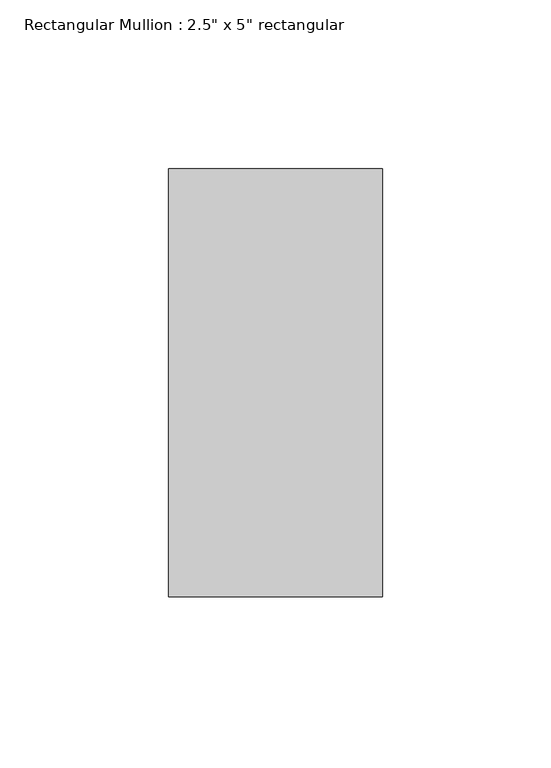
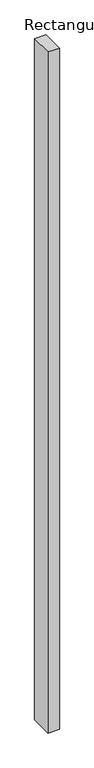
"""IFC4 building model written with IfcOpenShell, lengths in millimetres: member geometry."""

from ifc_helpers import new_model, si_unit, frame, origin, place, context, project, spatial, polyline, outline, extrude, source, transform, mapped, element, save


def member_7582bdd1(model_context):
    return source(origin(), model_context, "Body", "SweptSolid", [
        extrude(outline(polyline([(0.0, 63.5), (0.0, -63.5), (-63.5, -63.5), (-63.5, 63.5), (0.0, 63.5)])), frame((0.0, 0.0, -4003.9584783), z_axis=(0.0, 0.0, 1.0), x_axis=(1.0, 0.0, 0.0)), (0.0, 0.0, 1.0), 4003.9584783),
    ])


if __name__ == "__main__":
    model = new_model("IFC4")
    model_context = context("Model", 3, world=origin())
    ifc_project = project(units=[si_unit("LENGTHUNIT", "METRE", prefix="MILLI")], contexts=[model_context])
    site = spatial("IfcSite", under=ifc_project)
    building = spatial("IfcBuilding", under=site)
    placement = place(None, origin())
    member_shape = member_7582bdd1(model_context)
    element("IfcMember", 1, ObjectType="Rectangular Mullion : 2.5\" x 5\" rectangular", at=placement, inside=building, context=model_context, shape_type="MappedRepresentation", body=[
        mapped(member_shape, transform((0.0, 0.0, 0.0), x_axis=(1.0, 0.0, 0.0), y_axis=(0.0, 1.0, 0.0), z_axis=(0.0, 0.0, 1.0))),
    ])
    save(model, "model.ifc")

# Revit data of these elements
# Type "Rectangular Mullion : 2.5\" x 5\" rectangular"
#   built-in parameter 1007304 = 0.416667 (stored number, unit not read)
#   built-in parameter 1007301 = 0.104167 (stored number, unit not read)
#   built-in parameter 1007300 = 0.104167 (stored number, unit not read)
# Element 1 (IfcMember, "Rectangular Mullion : 2.5\" x 5\" rectangular")
#   Materials on its faces: "Iron, Ductile"
# Materials
#   "Iron, Ductile": class "Metal", colour RGB 0 0 0, transparency 0, Description = "Ductile cast iron", Cost = 0
